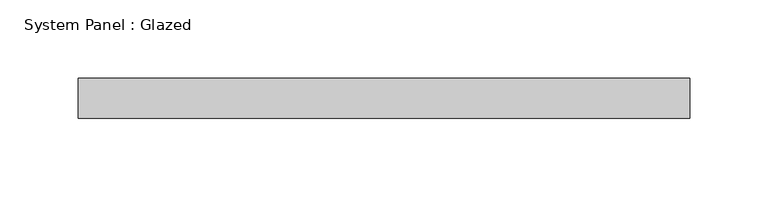
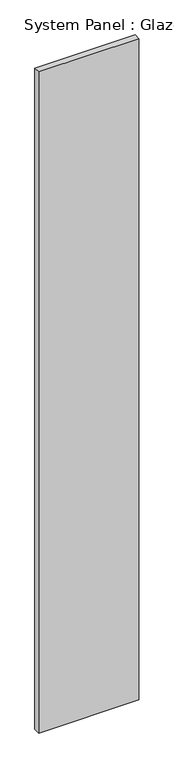
"""IFC4 building model written with IfcOpenShell, lengths in millimetres: plate geometry, System Panel : Glazed."""

from ifc_helpers import new_model, si_unit, origin, origin_with_axes, place, context, project, spatial, polyline, outline, extrude, source, transform, mapped, element, save


def system_panel_glazed_7e745cad(model_context):
    return source(origin(), model_context, "Body", "SweptSolid", [
        extrude(outline(polyline([(194.7333333, 19.05), (-194.7333333, 19.05), (-194.7333333, 44.45), (194.7333333, 44.45), (194.7333333, 19.05)])), origin_with_axes(), (0.0, 0.0, 1.0), 2719.788773),
    ])


if __name__ == "__main__":
    model = new_model("IFC4")
    model_context = context("Model", 3, world=origin())
    ifc_project = project(units=[si_unit("LENGTHUNIT", "METRE", prefix="MILLI")], contexts=[model_context])
    site = spatial("IfcSite", under=ifc_project)
    building = spatial("IfcBuilding", under=site)
    placement = place(None, origin())
    system_panel_glazed_shape = system_panel_glazed_7e745cad(model_context)
    element("IfcPlate", 1, ObjectType="System Panel : Glazed", at=placement, inside=building, context=model_context, shape_type="MappedRepresentation", body=[
        mapped(system_panel_glazed_shape, transform((0.0, 0.0, 0.0), x_axis=(1.0, 0.0, 0.0), y_axis=(0.0, 1.0, 0.0), z_axis=(0.0, 0.0, 1.0))),
    ])
    save(model, "model.ifc")

# Revit data of these elements
# Type "System Panel : Glazed"
#   Construction Type Id = "GSP4R"
#   Analytic Construction = "1/8 in Pilkington single glazing"
#   Visual Light Transmittance = 0.9
#   Solar Heat Gain Coefficient = 0.86
#   Heat Transfer Coefficient (U) = 1.18115 BTU/(h·ft²·°F)
# Element 1 (IfcPlate, "System Panel : Glazed")
#   Materials on its faces: "Glass"
# Materials
#   "Glass": class "Glass", colour RGB 0 128 192, transparency 0.75, Description = "Soda Lime Glass", Cost = 0
